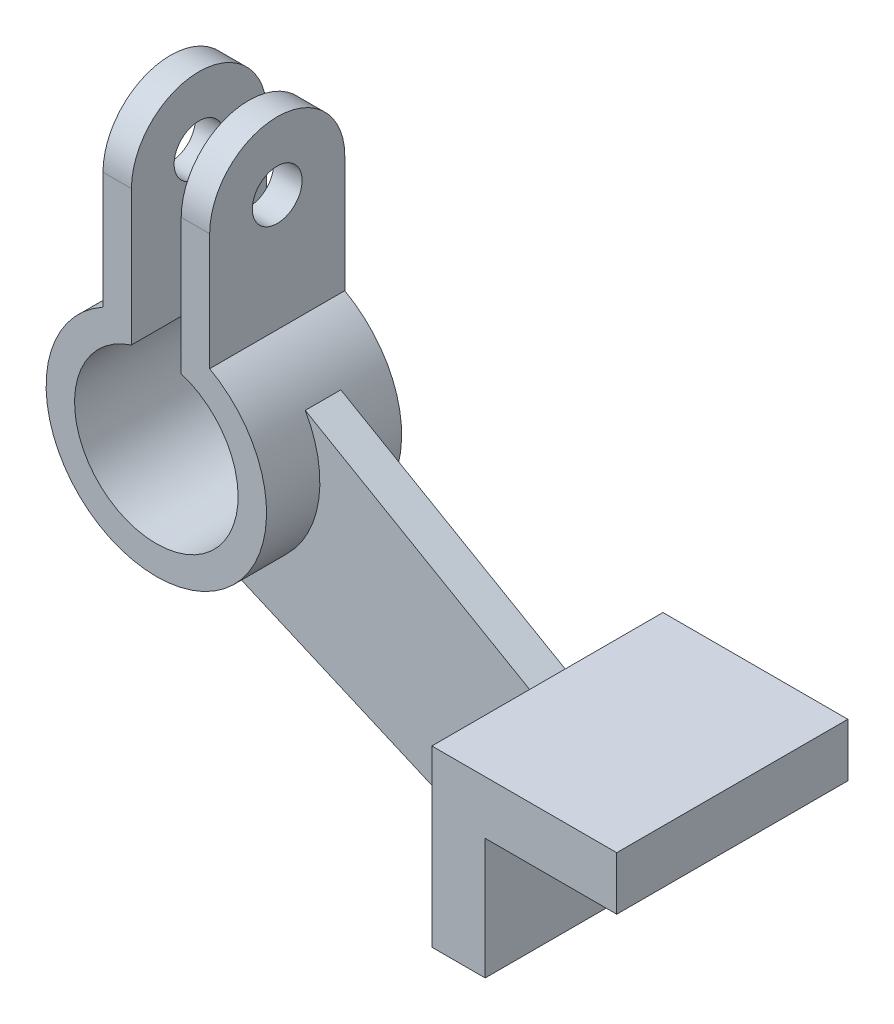
ISO-10303-21;
HEADER;
FILE_DESCRIPTION(('STEP AP214'),'2;1');
FILE_NAME('part.step','',(''),(''),'','','');
FILE_SCHEMA(('AUTOMOTIVE_DESIGN { 1 0 10303 214 1 1 1 1 }'));
ENDSEC;
DATA;
#1=APPLICATION_CONTEXT('core data for automotive mechanical design processes');
#2=APPLICATION_PROTOCOL_DEFINITION('international standard','automotive_design',2000,#1);
#3=PRODUCT_CONTEXT('',#1,'mechanical');
#4=PRODUCT('Part','Part','',(#3));
#5=PRODUCT_RELATED_PRODUCT_CATEGORY('part','',(#4));
#6=PRODUCT_DEFINITION_FORMATION('','',#4);
#7=PRODUCT_DEFINITION_CONTEXT('part definition',#1,'design');
#8=PRODUCT_DEFINITION('design','',#6,#7);
#9=PRODUCT_DEFINITION_SHAPE('','',#8);
#10=(LENGTH_UNIT() NAMED_UNIT(*) SI_UNIT(.MILLI.,.METRE.));
#11=(NAMED_UNIT(*) PLANE_ANGLE_UNIT() SI_UNIT($,.RADIAN.));
#12=(NAMED_UNIT(*) SI_UNIT($,.STERADIAN.) SOLID_ANGLE_UNIT());
#13=UNCERTAINTY_MEASURE_WITH_UNIT(LENGTH_MEASURE(1.E-05),#10,'distance_accuracy_value','');
#14=(GEOMETRIC_REPRESENTATION_CONTEXT(3) GLOBAL_UNCERTAINTY_ASSIGNED_CONTEXT((#13)) GLOBAL_UNIT_ASSIGNED_CONTEXT((#10,
#11,#12)) REPRESENTATION_CONTEXT('',''));
#15=CARTESIAN_POINT('',(0.,0.,0.));
#16=DIRECTION('',(0.,0.,1.));
#17=DIRECTION('',(1.,0.,0.));
#18=AXIS2_PLACEMENT_3D('',#15,#16,#17);
#19=CARTESIAN_POINT('',(-2.61943244872498E-13,1.4658413372004E-13,23.));
#20=DIRECTION('',(0.,0.,-1.));
#21=DIRECTION('',(-1.,0.,0.));
#22=AXIS2_PLACEMENT_3D('',#19,#20,#21);
#23=PLANE('',#22);
#24=DIRECTION('',(0.,-1.,0.));
#25=VECTOR('',#24,1.);
#26=CARTESIAN_POINT('',(90.,1.4658413372004E-13,23.));
#27=LINE('',#26,#25);
#28=CARTESIAN_POINT('',(90.,-21.0099338120634,23.));
#29=VERTEX_POINT('',#28);
#30=CARTESIAN_POINT('',(90.,-70.0360003093009,23.));
#31=VERTEX_POINT('',#30);
#32=EDGE_CURVE('E192',#29,#31,#27,.T.);
#33=ORIENTED_EDGE('',*,*,#32,.F.);
#34=DIRECTION('',(-0.86602540378444,0.499999999999998,0.));
#35=VECTOR('',#34,1.);
#36=CARTESIAN_POINT('',(90.,-21.0099338120634,23.));
#37=LINE('',#36,#35);
#38=CARTESIAN_POINT('',(26.888515956955,15.4274984891452,23.));
#39=VERTEX_POINT('',#38);
#40=EDGE_CURVE('E201',#29,#39,#37,.T.);
#41=ORIENTED_EDGE('',*,*,#40,.T.);
#42=CARTESIAN_POINT('',(-2.61943244872498E-13,1.4658413372004E-13,23.));
#43=DIRECTION('',(0.,0.,-1.));
#44=DIRECTION('',(-1.,0.,0.));
#45=AXIS2_PLACEMENT_3D('',#42,#43,#44);
#46=CIRCLE('',#45,31.0000000000002);
#47=CARTESIAN_POINT('',(0.,-31.,23.));
#48=VERTEX_POINT('',#47);
#49=EDGE_CURVE('E202',#39,#48,#46,.T.);
#50=ORIENTED_EDGE('',*,*,#49,.T.);
#51=DIRECTION('',(0.917421692084343,-0.397916371732931,0.));
#52=VECTOR('',#51,1.);
#53=CARTESIAN_POINT('',(90.,-70.0360003093009,23.));
#54=LINE('',#53,#52);
#55=EDGE_CURVE('E210',#48,#31,#54,.T.);
#56=ORIENTED_EDGE('',*,*,#55,.T.);
#57=EDGE_LOOP('',(#33,#41,#50,#56));
#58=FACE_BOUND('',#57,.T.);
#59=ADVANCED_FACE('F41',(#58),#23,.F.);
#60=CARTESIAN_POINT('',(-2.61943244872498E-13,1.4658413372004E-13,13.));
#61=DIRECTION('',(0.,0.,-1.));
#62=DIRECTION('',(-1.,0.,0.));
#63=AXIS2_PLACEMENT_3D('',#60,#61,#62);
#64=PLANE('',#63);
#65=DIRECTION('',(-0.86602540378444,0.499999999999998,0.));
#66=VECTOR('',#65,1.);
#67=CARTESIAN_POINT('',(90.,-21.0099338120634,13.));
#68=LINE('',#67,#66);
#69=CARTESIAN_POINT('',(90.,-21.0099338120634,13.));
#70=VERTEX_POINT('',#69);
#71=CARTESIAN_POINT('',(26.888515956955,15.4274984891452,13.));
#72=VERTEX_POINT('',#71);
#73=EDGE_CURVE('E197',#70,#72,#68,.T.);
#74=ORIENTED_EDGE('',*,*,#73,.F.);
#75=DIRECTION('',(0.,-1.,0.));
#76=VECTOR('',#75,1.);
#77=CARTESIAN_POINT('',(90.,1.4658413372004E-13,13.));
#78=LINE('',#77,#76);
#79=CARTESIAN_POINT('',(90.,-70.0360003093009,13.));
#80=VERTEX_POINT('',#79);
#81=EDGE_CURVE('E11',#70,#80,#78,.T.);
#82=ORIENTED_EDGE('',*,*,#81,.T.);
#83=DIRECTION('',(0.917421692084343,-0.397916371732931,0.));
#84=VECTOR('',#83,1.);
#85=CARTESIAN_POINT('',(90.,-70.0360003093009,13.));
#86=LINE('',#85,#84);
#87=CARTESIAN_POINT('',(0.,-31.,13.));
#88=VERTEX_POINT('',#87);
#89=EDGE_CURVE('E54',#88,#80,#86,.T.);
#90=ORIENTED_EDGE('',*,*,#89,.F.);
#91=CARTESIAN_POINT('',(-2.61943244872498E-13,1.4658413372004E-13,13.));
#92=DIRECTION('',(0.,0.,-1.));
#93=DIRECTION('',(-1.,0.,0.));
#94=AXIS2_PLACEMENT_3D('',#91,#92,#93);
#95=CIRCLE('',#94,31.0000000000002);
#96=EDGE_CURVE('E211',#72,#88,#95,.T.);
#97=ORIENTED_EDGE('',*,*,#96,.F.);
#98=EDGE_LOOP('',(#74,#82,#90,#97));
#99=FACE_BOUND('',#98,.T.);
#100=ADVANCED_FACE('F352',(#99),#64,.T.);
#101=CARTESIAN_POINT('',(0.,0.,38.));
#102=DIRECTION('',(0.,0.,-1.));
#103=DIRECTION('',(-1.,0.,0.));
#104=AXIS2_PLACEMENT_3D('',#101,#102,#103);
#105=CYLINDRICAL_SURFACE('',#104,31.);
#106=CARTESIAN_POINT('',(0.,0.,38.));
#107=DIRECTION('',(0.,0.,1.));
#108=DIRECTION('',(1.,0.,0.));
#109=AXIS2_PLACEMENT_3D('',#106,#107,#108);
#110=CIRCLE('',#109,31.);
#111=CARTESIAN_POINT('',(-15.,27.1293199325011,38.));
#112=VERTEX_POINT('',#111);
#113=CARTESIAN_POINT('',(15.,27.1293199325011,38.));
#114=VERTEX_POINT('',#113);
#115=EDGE_CURVE('E65',#112,#114,#110,.T.);
#116=ORIENTED_EDGE('',*,*,#115,.F.);
#117=DIRECTION('',(0.,0.,-1.));
#118=VECTOR('',#117,1.);
#119=CARTESIAN_POINT('',(-15.,27.1293199325011,38.));
#120=LINE('',#119,#118);
#121=CARTESIAN_POINT('',(-15.,27.1293199325011,0.));
#122=VERTEX_POINT('',#121);
#123=EDGE_CURVE('E47',#112,#122,#120,.T.);
#124=ORIENTED_EDGE('',*,*,#123,.T.);
#125=CARTESIAN_POINT('',(0.,0.,0.));
#126=DIRECTION('',(0.,0.,1.));
#127=DIRECTION('',(1.,0.,0.));
#128=AXIS2_PLACEMENT_3D('',#125,#126,#127);
#129=CIRCLE('',#128,31.);
#130=CARTESIAN_POINT('',(15.,27.1293199325011,0.));
#131=VERTEX_POINT('',#130);
#132=EDGE_CURVE('E289',#122,#131,#129,.T.);
#133=ORIENTED_EDGE('',*,*,#132,.T.);
#134=DIRECTION('',(0.,0.,-1.));
#135=VECTOR('',#134,1.);
#136=CARTESIAN_POINT('',(15.,27.1293199325011,38.));
#137=LINE('',#136,#135);
#138=EDGE_CURVE('E296',#131,#114,#137,.F.);
#139=ORIENTED_EDGE('',*,*,#138,.T.);
#140=EDGE_LOOP('',(#116,#124,#133,#139));
#141=FACE_BOUND('',#140,.T.);
#142=ORIENTED_EDGE('',*,*,#49,.F.);
#143=DIRECTION('',(0.,0.,-1.));
#144=VECTOR('',#143,1.);
#145=CARTESIAN_POINT('',(26.888515956955,15.4274984891452,23.));
#146=LINE('',#145,#144);
#147=EDGE_CURVE('E217',#39,#72,#146,.T.);
#148=ORIENTED_EDGE('',*,*,#147,.T.);
#149=ORIENTED_EDGE('',*,*,#96,.T.);
#150=DIRECTION('',(0.,0.,-1.));
#151=VECTOR('',#150,1.);
#152=CARTESIAN_POINT('',(0.,-31.,23.));
#153=LINE('',#152,#151);
#154=EDGE_CURVE('E216',#48,#88,#153,.T.);
#155=ORIENTED_EDGE('',*,*,#154,.F.);
#156=EDGE_LOOP('',(#142,#148,#149,#155));
#157=FACE_BOUND('',#156,.T.);
#158=ADVANCED_FACE('F43',(#141,#157),#105,.T.);
#159=CARTESIAN_POINT('',(0.,0.,38.));
#160=DIRECTION('',(0.,0.,1.));
#161=DIRECTION('',(1.,0.,0.));
#162=AXIS2_PLACEMENT_3D('',#159,#160,#161);
#163=PLANE('',#162);
#164=CARTESIAN_POINT('',(0.,0.,38.));
#165=DIRECTION('',(0.,0.,1.));
#166=DIRECTION('',(1.,0.,0.));
#167=AXIS2_PLACEMENT_3D('',#164,#165,#166);
#168=CIRCLE('',#167,23.);
#169=CARTESIAN_POINT('',(-7.,21.9089023002066,38.));
#170=VERTEX_POINT('',#169);
#171=CARTESIAN_POINT('',(7.,21.9089023002066,38.));
#172=VERTEX_POINT('',#171);
#173=EDGE_CURVE('E290',#170,#172,#168,.T.);
#174=ORIENTED_EDGE('',*,*,#173,.F.);
#175=DIRECTION('',(0.,-1.,0.));
#176=VECTOR('',#175,1.);
#177=CARTESIAN_POINT('',(-7.,0.,38.));
#178=LINE('',#177,#176);
#179=CARTESIAN_POINT('',(-7.,60.,38.));
#180=VERTEX_POINT('',#179);
#181=EDGE_CURVE('E282',#180,#170,#178,.T.);
#182=ORIENTED_EDGE('',*,*,#181,.F.);
#183=DIRECTION('',(1.,0.,0.));
#184=VECTOR('',#183,1.);
#185=CARTESIAN_POINT('',(-15.,60.,38.));
#186=LINE('',#185,#184);
#187=CARTESIAN_POINT('',(-15.,60.,38.));
#188=VERTEX_POINT('',#187);
#189=EDGE_CURVE('E248',#188,#180,#186,.T.);
#190=ORIENTED_EDGE('',*,*,#189,.F.);
#191=DIRECTION('',(0.,-1.,0.));
#192=VECTOR('',#191,1.);
#193=CARTESIAN_POINT('',(-15.,60.,38.));
#194=LINE('',#193,#192);
#195=EDGE_CURVE('E245',#188,#112,#194,.T.);
#196=ORIENTED_EDGE('',*,*,#195,.T.);
#197=ORIENTED_EDGE('',*,*,#115,.T.);
#198=DIRECTION('',(0.,-1.,0.));
#199=VECTOR('',#198,1.);
#200=CARTESIAN_POINT('',(15.,60.,38.));
#201=LINE('',#200,#199);
#202=CARTESIAN_POINT('',(15.,60.,38.));
#203=VERTEX_POINT('',#202);
#204=EDGE_CURVE('E262',#203,#114,#201,.T.);
#205=ORIENTED_EDGE('',*,*,#204,.F.);
#206=DIRECTION('',(-1.,0.,0.));
#207=VECTOR('',#206,1.);
#208=CARTESIAN_POINT('',(15.,60.,38.));
#209=LINE('',#208,#207);
#210=CARTESIAN_POINT('',(7.,60.,38.));
#211=VERTEX_POINT('',#210);
#212=EDGE_CURVE('E273',#203,#211,#209,.T.);
#213=ORIENTED_EDGE('',*,*,#212,.T.);
#214=DIRECTION('',(0.,1.,0.));
#215=VECTOR('',#214,1.);
#216=CARTESIAN_POINT('',(7.,0.,38.));
#217=LINE('',#216,#215);
#218=EDGE_CURVE('E280',#172,#211,#217,.T.);
#219=ORIENTED_EDGE('',*,*,#218,.F.);
#220=EDGE_LOOP('',(#174,#182,#190,#196,#197,#205,#213,#219));
#221=FACE_BOUND('',#220,.T.);
#222=ADVANCED_FACE('F328',(#221),#163,.T.);
#223=CARTESIAN_POINT('',(0.,0.,0.));
#224=DIRECTION('',(0.,0.,1.));
#225=DIRECTION('',(1.,0.,0.));
#226=AXIS2_PLACEMENT_3D('',#223,#224,#225);
#227=PLANE('',#226);
#228=DIRECTION('',(0.,-1.,0.));
#229=VECTOR('',#228,1.);
#230=CARTESIAN_POINT('',(-7.,0.,0.));
#231=LINE('',#230,#229);
#232=CARTESIAN_POINT('',(-7.,60.,0.));
#233=VERTEX_POINT('',#232);
#234=CARTESIAN_POINT('',(-7.,21.9089023002066,0.));
#235=VERTEX_POINT('',#234);
#236=EDGE_CURVE('E278',#233,#235,#231,.T.);
#237=ORIENTED_EDGE('',*,*,#236,.T.);
#238=CARTESIAN_POINT('',(0.,0.,0.));
#239=DIRECTION('',(0.,0.,1.));
#240=DIRECTION('',(1.,0.,0.));
#241=AXIS2_PLACEMENT_3D('',#238,#239,#240);
#242=CIRCLE('',#241,23.);
#243=CARTESIAN_POINT('',(7.,21.9089023002066,0.));
#244=VERTEX_POINT('',#243);
#245=EDGE_CURVE('E281',#235,#244,#242,.T.);
#246=ORIENTED_EDGE('',*,*,#245,.T.);
#247=DIRECTION('',(0.,1.,0.));
#248=VECTOR('',#247,1.);
#249=CARTESIAN_POINT('',(7.,0.,0.));
#250=LINE('',#249,#248);
#251=CARTESIAN_POINT('',(7.,60.,0.));
#252=VERTEX_POINT('',#251);
#253=EDGE_CURVE('E279',#244,#252,#250,.T.);
#254=ORIENTED_EDGE('',*,*,#253,.T.);
#255=DIRECTION('',(-1.,0.,0.));
#256=VECTOR('',#255,1.);
#257=CARTESIAN_POINT('',(15.,60.,0.));
#258=LINE('',#257,#256);
#259=CARTESIAN_POINT('',(15.,60.,0.));
#260=VERTEX_POINT('',#259);
#261=EDGE_CURVE('E267',#260,#252,#258,.T.);
#262=ORIENTED_EDGE('',*,*,#261,.F.);
#263=DIRECTION('',(0.,1.,0.));
#264=VECTOR('',#263,1.);
#265=CARTESIAN_POINT('',(15.,21.9089023002066,0.));
#266=LINE('',#265,#264);
#267=EDGE_CURVE('E270',#131,#260,#266,.T.);
#268=ORIENTED_EDGE('',*,*,#267,.F.);
#269=ORIENTED_EDGE('',*,*,#132,.F.);
#270=DIRECTION('',(0.,1.,0.));
#271=VECTOR('',#270,1.);
#272=CARTESIAN_POINT('',(-15.,21.9089023002066,0.));
#273=LINE('',#272,#271);
#274=CARTESIAN_POINT('',(-15.,60.,0.));
#275=VERTEX_POINT('',#274);
#276=EDGE_CURVE('E242',#122,#275,#273,.T.);
#277=ORIENTED_EDGE('',*,*,#276,.T.);
#278=DIRECTION('',(1.,0.,0.));
#279=VECTOR('',#278,1.);
#280=CARTESIAN_POINT('',(-15.,60.,0.));
#281=LINE('',#280,#279);
#282=EDGE_CURVE('E253',#275,#233,#281,.T.);
#283=ORIENTED_EDGE('',*,*,#282,.T.);
#284=EDGE_LOOP('',(#237,#246,#254,#262,#268,#269,#277,#283));
#285=FACE_BOUND('',#284,.T.);
#286=ADVANCED_FACE('F306',(#285),#227,.F.);
#287=CARTESIAN_POINT('',(0.,0.,38.));
#288=DIRECTION('',(0.,0.,-1.));
#289=DIRECTION('',(-1.,0.,0.));
#290=AXIS2_PLACEMENT_3D('',#287,#288,#289);
#291=CYLINDRICAL_SURFACE('',#290,23.);
#292=DIRECTION('',(0.,0.,-1.));
#293=VECTOR('',#292,1.);
#294=CARTESIAN_POINT('',(-7.,21.9089023002066,38.));
#295=LINE('',#294,#293);
#296=EDGE_CURVE('E299',#170,#235,#295,.T.);
#297=ORIENTED_EDGE('',*,*,#296,.F.);
#298=ORIENTED_EDGE('',*,*,#173,.T.);
#299=DIRECTION('',(0.,0.,-1.));
#300=VECTOR('',#299,1.);
#301=CARTESIAN_POINT('',(7.,21.9089023002066,38.));
#302=LINE('',#301,#300);
#303=EDGE_CURVE('E294',#244,#172,#302,.F.);
#304=ORIENTED_EDGE('',*,*,#303,.F.);
#305=ORIENTED_EDGE('',*,*,#245,.F.);
#306=EDGE_LOOP('',(#297,#298,#304,#305));
#307=FACE_BOUND('',#306,.T.);
#308=ADVANCED_FACE('F321',(#307),#291,.F.);
#309=CARTESIAN_POINT('',(7.,0.,0.));
#310=DIRECTION('',(1.,0.,0.));
#311=DIRECTION('',(0.,0.,-1.));
#312=AXIS2_PLACEMENT_3D('',#309,#310,#311);
#313=PLANE('',#312);
#314=ORIENTED_EDGE('',*,*,#253,.F.);
#315=ORIENTED_EDGE('',*,*,#303,.T.);
#316=ORIENTED_EDGE('',*,*,#218,.T.);
#317=CARTESIAN_POINT('',(7.,60.,19.));
#318=DIRECTION('',(1.,0.,0.));
#319=DIRECTION('',(0.,0.,-1.));
#320=AXIS2_PLACEMENT_3D('',#317,#318,#319);
#321=CIRCLE('',#320,19.);
#322=EDGE_CURVE('E256',#252,#211,#321,.T.);
#323=ORIENTED_EDGE('',*,*,#322,.F.);
#324=EDGE_LOOP('',(#314,#315,#316,#323));
#325=FACE_BOUND('',#324,.T.);
#326=CARTESIAN_POINT('',(7.,60.,19.));
#327=DIRECTION('',(1.,0.,0.));
#328=DIRECTION('',(0.,0.,-1.));
#329=AXIS2_PLACEMENT_3D('',#326,#327,#328);
#330=CIRCLE('',#329,7.);
#331=CARTESIAN_POINT('',(7.,60.,12.));
#332=VERTEX_POINT('',#331);
#333=EDGE_CURVE('E255',#332,#332,#330,.T.);
#334=ORIENTED_EDGE('',*,*,#333,.T.);
#335=EDGE_LOOP('',(#334));
#336=FACE_BOUND('',#335,.T.);
#337=ADVANCED_FACE('F324',(#325,#336),#313,.F.);
#338=CARTESIAN_POINT('',(-7.,0.,0.));
#339=DIRECTION('',(-1.,0.,0.));
#340=DIRECTION('',(0.,0.,1.));
#341=AXIS2_PLACEMENT_3D('',#338,#339,#340);
#342=PLANE('',#341);
#343=ORIENTED_EDGE('',*,*,#181,.T.);
#344=ORIENTED_EDGE('',*,*,#296,.T.);
#345=ORIENTED_EDGE('',*,*,#236,.F.);
#346=CARTESIAN_POINT('',(-7.,60.,19.));
#347=DIRECTION('',(1.,0.,0.));
#348=DIRECTION('',(0.,0.,-1.));
#349=AXIS2_PLACEMENT_3D('',#346,#347,#348);
#350=CIRCLE('',#349,19.);
#351=EDGE_CURVE('E234',#233,#180,#350,.T.);
#352=ORIENTED_EDGE('',*,*,#351,.T.);
#353=EDGE_LOOP('',(#343,#344,#345,#352));
#354=FACE_BOUND('',#353,.T.);
#355=CARTESIAN_POINT('',(-7.,60.,19.));
#356=DIRECTION('',(1.,0.,0.));
#357=DIRECTION('',(0.,0.,-1.));
#358=AXIS2_PLACEMENT_3D('',#355,#356,#357);
#359=CIRCLE('',#358,7.);
#360=CARTESIAN_POINT('',(-7.,60.,12.));
#361=VERTEX_POINT('',#360);
#362=EDGE_CURVE('E233',#361,#361,#359,.T.);
#363=ORIENTED_EDGE('',*,*,#362,.F.);
#364=EDGE_LOOP('',(#363));
#365=FACE_BOUND('',#364,.T.);
#366=ADVANCED_FACE('F339',(#354,#365),#342,.F.);
#367=CARTESIAN_POINT('',(15.,60.,19.));
#368=DIRECTION('',(1.,0.,0.));
#369=DIRECTION('',(0.,0.,-1.));
#370=AXIS2_PLACEMENT_3D('',#367,#368,#369);
#371=PLANE('',#370);
#372=CARTESIAN_POINT('',(15.,60.,19.));
#373=DIRECTION('',(1.,0.,0.));
#374=DIRECTION('',(0.,0.,-1.));
#375=AXIS2_PLACEMENT_3D('',#372,#373,#374);
#376=CIRCLE('',#375,7.);
#377=CARTESIAN_POINT('',(15.,60.,12.));
#378=VERTEX_POINT('',#377);
#379=EDGE_CURVE('E254',#378,#378,#376,.T.);
#380=ORIENTED_EDGE('',*,*,#379,.F.);
#381=EDGE_LOOP('',(#380));
#382=FACE_BOUND('',#381,.T.);
#383=ORIENTED_EDGE('',*,*,#138,.F.);
#384=ORIENTED_EDGE('',*,*,#267,.T.);
#385=CARTESIAN_POINT('',(15.,60.,19.));
#386=DIRECTION('',(1.,0.,0.));
#387=DIRECTION('',(0.,0.,-1.));
#388=AXIS2_PLACEMENT_3D('',#385,#386,#387);
#389=CIRCLE('',#388,19.);
#390=EDGE_CURVE('E261',#260,#203,#389,.T.);
#391=ORIENTED_EDGE('',*,*,#390,.T.);
#392=ORIENTED_EDGE('',*,*,#204,.T.);
#393=EDGE_LOOP('',(#383,#384,#391,#392));
#394=FACE_BOUND('',#393,.T.);
#395=ADVANCED_FACE('F333',(#382,#394),#371,.T.);
#396=CARTESIAN_POINT('',(15.,60.,19.));
#397=DIRECTION('',(-1.,0.,0.));
#398=DIRECTION('',(0.,0.,1.));
#399=AXIS2_PLACEMENT_3D('',#396,#397,#398);
#400=CYLINDRICAL_SURFACE('',#399,19.);
#401=ORIENTED_EDGE('',*,*,#322,.T.);
#402=ORIENTED_EDGE('',*,*,#212,.F.);
#403=ORIENTED_EDGE('',*,*,#390,.F.);
#404=ORIENTED_EDGE('',*,*,#261,.T.);
#405=EDGE_LOOP('',(#401,#402,#403,#404));
#406=FACE_BOUND('',#405,.T.);
#407=ADVANCED_FACE('F334',(#406),#400,.T.);
#408=CARTESIAN_POINT('',(15.,60.,19.));
#409=DIRECTION('',(-1.,0.,0.));
#410=DIRECTION('',(0.,0.,1.));
#411=AXIS2_PLACEMENT_3D('',#408,#409,#410);
#412=CYLINDRICAL_SURFACE('',#411,7.);
#413=ORIENTED_EDGE('',*,*,#379,.T.);
#414=EDGE_LOOP('',(#413));
#415=FACE_BOUND('',#414,.T.);
#416=ORIENTED_EDGE('',*,*,#333,.F.);
#417=EDGE_LOOP('',(#416));
#418=FACE_BOUND('',#417,.T.);
#419=ADVANCED_FACE('F342',(#415,#418),#412,.F.);
#420=CARTESIAN_POINT('',(-15.,60.,19.));
#421=DIRECTION('',(-1.,0.,0.));
#422=DIRECTION('',(0.,0.,-1.));
#423=AXIS2_PLACEMENT_3D('',#420,#421,#422);
#424=PLANE('',#423);
#425=CARTESIAN_POINT('',(-15.,60.,19.));
#426=DIRECTION('',(1.,0.,0.));
#427=DIRECTION('',(0.,0.,-1.));
#428=AXIS2_PLACEMENT_3D('',#425,#426,#427);
#429=CIRCLE('',#428,7.);
#430=CARTESIAN_POINT('',(-15.,60.,12.));
#431=VERTEX_POINT('',#430);
#432=EDGE_CURVE('E235',#431,#431,#429,.T.);
#433=ORIENTED_EDGE('',*,*,#432,.T.);
#434=EDGE_LOOP('',(#433));
#435=FACE_BOUND('',#434,.T.);
#436=ORIENTED_EDGE('',*,*,#123,.F.);
#437=ORIENTED_EDGE('',*,*,#195,.F.);
#438=CARTESIAN_POINT('',(-15.,60.,19.));
#439=DIRECTION('',(1.,0.,0.));
#440=DIRECTION('',(0.,0.,-1.));
#441=AXIS2_PLACEMENT_3D('',#438,#439,#440);
#442=CIRCLE('',#441,19.);
#443=EDGE_CURVE('E236',#275,#188,#442,.T.);
#444=ORIENTED_EDGE('',*,*,#443,.F.);
#445=ORIENTED_EDGE('',*,*,#276,.F.);
#446=EDGE_LOOP('',(#436,#437,#444,#445));
#447=FACE_BOUND('',#446,.T.);
#448=ADVANCED_FACE('F315',(#435,#447),#424,.T.);
#449=CARTESIAN_POINT('',(-15.,60.,19.));
#450=DIRECTION('',(1.,0.,0.));
#451=DIRECTION('',(0.,0.,-1.));
#452=AXIS2_PLACEMENT_3D('',#449,#450,#451);
#453=CYLINDRICAL_SURFACE('',#452,19.);
#454=ORIENTED_EDGE('',*,*,#351,.F.);
#455=ORIENTED_EDGE('',*,*,#282,.F.);
#456=ORIENTED_EDGE('',*,*,#443,.T.);
#457=ORIENTED_EDGE('',*,*,#189,.T.);
#458=EDGE_LOOP('',(#454,#455,#456,#457));
#459=FACE_BOUND('',#458,.T.);
#460=ADVANCED_FACE('F312',(#459),#453,.T.);
#461=CARTESIAN_POINT('',(-15.,60.,19.));
#462=DIRECTION('',(1.,0.,0.));
#463=DIRECTION('',(0.,0.,-1.));
#464=AXIS2_PLACEMENT_3D('',#461,#462,#463);
#465=CYLINDRICAL_SURFACE('',#464,7.);
#466=ORIENTED_EDGE('',*,*,#432,.F.);
#467=EDGE_LOOP('',(#466));
#468=FACE_BOUND('',#467,.T.);
#469=ORIENTED_EDGE('',*,*,#362,.T.);
#470=EDGE_LOOP('',(#469));
#471=FACE_BOUND('',#470,.T.);
#472=ADVANCED_FACE('F388',(#468,#471),#465,.F.);
#473=CARTESIAN_POINT('',(90.,-70.0360003093009,23.));
#474=DIRECTION('',(0.,1.,0.));
#475=DIRECTION('',(0.,0.,1.));
#476=AXIS2_PLACEMENT_3D('',#473,#474,#475);
#477=PLANE('',#476);
#478=DIRECTION('',(0.,0.,-1.));
#479=VECTOR('',#478,1.);
#480=CARTESIAN_POINT('',(90.,-70.0360003093009,23.));
#481=LINE('',#480,#479);
#482=EDGE_CURVE('E207',#31,#80,#481,.T.);
#483=ORIENTED_EDGE('',*,*,#482,.T.);
#484=DIRECTION('',(0.,0.,-1.));
#485=VECTOR('',#484,1.);
#486=CARTESIAN_POINT('',(90.,-70.0360003093009,50.5));
#487=LINE('',#486,#485);
#488=CARTESIAN_POINT('',(90.,-70.0360003093009,-14.5));
#489=VERTEX_POINT('',#488);
#490=EDGE_CURVE('E194',#80,#489,#487,.T.);
#491=ORIENTED_EDGE('',*,*,#490,.T.);
#492=DIRECTION('',(1.,0.,0.));
#493=VECTOR('',#492,1.);
#494=CARTESIAN_POINT('',(90.,-70.0360003093009,-14.5));
#495=LINE('',#494,#493);
#496=CARTESIAN_POINT('',(105.,-70.0360003093009,-14.5));
#497=VERTEX_POINT('',#496);
#498=EDGE_CURVE('E555',#489,#497,#495,.T.);
#499=ORIENTED_EDGE('',*,*,#498,.T.);
#500=DIRECTION('',(0.,0.,-1.));
#501=VECTOR('',#500,1.);
#502=CARTESIAN_POINT('',(105.,-70.0360003093009,23.));
#503=LINE('',#502,#501);
#504=CARTESIAN_POINT('',(105.,-70.0360003093009,50.5));
#505=VERTEX_POINT('',#504);
#506=EDGE_CURVE('E171',#505,#497,#503,.T.);
#507=ORIENTED_EDGE('',*,*,#506,.F.);
#508=DIRECTION('',(1.,0.,0.));
#509=VECTOR('',#508,1.);
#510=CARTESIAN_POINT('',(90.,-70.0360003093009,50.5));
#511=LINE('',#510,#509);
#512=CARTESIAN_POINT('',(90.,-70.0360003093009,50.5));
#513=VERTEX_POINT('',#512);
#514=EDGE_CURVE('E170',#513,#505,#511,.T.);
#515=ORIENTED_EDGE('',*,*,#514,.F.);
#516=EDGE_CURVE('E174',#513,#31,#487,.T.);
#517=ORIENTED_EDGE('',*,*,#516,.T.);
#518=EDGE_LOOP('',(#483,#491,#499,#507,#515,#517));
#519=FACE_BOUND('',#518,.T.);
#520=ADVANCED_FACE('F168',(#519),#477,.F.);
#521=CARTESIAN_POINT('',(105.,-70.0360003093009,23.));
#522=DIRECTION('',(-1.,0.,0.));
#523=DIRECTION('',(0.,-1.,0.));
#524=AXIS2_PLACEMENT_3D('',#521,#522,#523);
#525=PLANE('',#524);
#526=ORIENTED_EDGE('',*,*,#506,.T.);
#527=DIRECTION('',(0.,1.,0.));
#528=VECTOR('',#527,1.);
#529=CARTESIAN_POINT('',(105.,-36.0099338120634,-14.5));
#530=LINE('',#529,#528);
#531=CARTESIAN_POINT('',(105.,-36.0099338120634,-14.5));
#532=VERTEX_POINT('',#531);
#533=EDGE_CURVE('E551',#497,#532,#530,.T.);
#534=ORIENTED_EDGE('',*,*,#533,.T.);
#535=DIRECTION('',(0.,0.,-1.));
#536=VECTOR('',#535,1.);
#537=CARTESIAN_POINT('',(105.,-36.0099338120634,23.));
#538=LINE('',#537,#536);
#539=CARTESIAN_POINT('',(105.,-36.0099338120634,50.5));
#540=VERTEX_POINT('',#539);
#541=EDGE_CURVE('E230',#540,#532,#538,.T.);
#542=ORIENTED_EDGE('',*,*,#541,.F.);
#543=DIRECTION('',(0.,1.,0.));
#544=VECTOR('',#543,1.);
#545=CARTESIAN_POINT('',(105.,-36.0099338120634,50.5));
#546=LINE('',#545,#544);
#547=EDGE_CURVE('E176',#505,#540,#546,.T.);
#548=ORIENTED_EDGE('',*,*,#547,.F.);
#549=EDGE_LOOP('',(#526,#534,#542,#548));
#550=FACE_BOUND('',#549,.T.);
#551=ADVANCED_FACE('F382',(#550),#525,.F.);
#552=CARTESIAN_POINT('',(105.,-36.0099338120634,23.));
#553=DIRECTION('',(0.,1.,0.));
#554=DIRECTION('',(-1.,0.,0.));
#555=AXIS2_PLACEMENT_3D('',#552,#553,#554);
#556=PLANE('',#555);
#557=ORIENTED_EDGE('',*,*,#541,.T.);
#558=DIRECTION('',(1.,0.,0.));
#559=VECTOR('',#558,1.);
#560=CARTESIAN_POINT('',(142.,-36.0099338120634,-14.5));
#561=LINE('',#560,#559);
#562=CARTESIAN_POINT('',(142.,-36.0099338120634,-14.5));
#563=VERTEX_POINT('',#562);
#564=EDGE_CURVE('E563',#532,#563,#561,.T.);
#565=ORIENTED_EDGE('',*,*,#564,.T.);
#566=DIRECTION('',(0.,0.,-1.));
#567=VECTOR('',#566,1.);
#568=CARTESIAN_POINT('',(142.,-36.0099338120634,23.));
#569=LINE('',#568,#567);
#570=CARTESIAN_POINT('',(142.,-36.0099338120634,50.5));
#571=VERTEX_POINT('',#570);
#572=EDGE_CURVE('E227',#571,#563,#569,.T.);
#573=ORIENTED_EDGE('',*,*,#572,.F.);
#574=DIRECTION('',(1.,0.,0.));
#575=VECTOR('',#574,1.);
#576=CARTESIAN_POINT('',(142.,-36.0099338120634,50.5));
#577=LINE('',#576,#575);
#578=EDGE_CURVE('E575',#540,#571,#577,.T.);
#579=ORIENTED_EDGE('',*,*,#578,.F.);
#580=EDGE_LOOP('',(#557,#565,#573,#579));
#581=FACE_BOUND('',#580,.T.);
#582=ADVANCED_FACE('F377',(#581),#556,.F.);
#583=CARTESIAN_POINT('',(142.,-36.0099338120634,23.));
#584=DIRECTION('',(-1.,0.,0.));
#585=DIRECTION('',(0.,-1.,0.));
#586=AXIS2_PLACEMENT_3D('',#583,#584,#585);
#587=PLANE('',#586);
#588=ORIENTED_EDGE('',*,*,#572,.T.);
#589=DIRECTION('',(0.,1.,0.));
#590=VECTOR('',#589,1.);
#591=CARTESIAN_POINT('',(142.,-21.0099338120634,-14.5));
#592=LINE('',#591,#590);
#593=CARTESIAN_POINT('',(142.,-21.0099338120634,-14.5));
#594=VERTEX_POINT('',#593);
#595=EDGE_CURVE('E562',#563,#594,#592,.T.);
#596=ORIENTED_EDGE('',*,*,#595,.T.);
#597=DIRECTION('',(0.,0.,-1.));
#598=VECTOR('',#597,1.);
#599=CARTESIAN_POINT('',(142.,-21.0099338120634,23.));
#600=LINE('',#599,#598);
#601=CARTESIAN_POINT('',(142.,-21.0099338120634,50.5));
#602=VERTEX_POINT('',#601);
#603=EDGE_CURVE('E221',#602,#594,#600,.T.);
#604=ORIENTED_EDGE('',*,*,#603,.F.);
#605=DIRECTION('',(0.,1.,0.));
#606=VECTOR('',#605,1.);
#607=CARTESIAN_POINT('',(142.,-21.0099338120634,50.5));
#608=LINE('',#607,#606);
#609=EDGE_CURVE('E579',#571,#602,#608,.T.);
#610=ORIENTED_EDGE('',*,*,#609,.F.);
#611=EDGE_LOOP('',(#588,#596,#604,#610));
#612=FACE_BOUND('',#611,.T.);
#613=ADVANCED_FACE('F374',(#612),#587,.F.);
#614=CARTESIAN_POINT('',(142.,-21.0099338120634,23.));
#615=DIRECTION('',(0.,-1.,0.));
#616=DIRECTION('',(1.,0.,0.));
#617=AXIS2_PLACEMENT_3D('',#614,#615,#616);
#618=PLANE('',#617);
#619=ORIENTED_EDGE('',*,*,#603,.T.);
#620=DIRECTION('',(-1.,0.,0.));
#621=VECTOR('',#620,1.);
#622=CARTESIAN_POINT('',(90.,-21.0099338120634,-14.5));
#623=LINE('',#622,#621);
#624=CARTESIAN_POINT('',(90.,-21.0099338120634,-14.5));
#625=VERTEX_POINT('',#624);
#626=EDGE_CURVE('E186',#594,#625,#623,.T.);
#627=ORIENTED_EDGE('',*,*,#626,.T.);
#628=DIRECTION('',(0.,0.,-1.));
#629=VECTOR('',#628,1.);
#630=CARTESIAN_POINT('',(90.,-21.0099338120634,50.5));
#631=LINE('',#630,#629);
#632=EDGE_CURVE('E570',#70,#625,#631,.T.);
#633=ORIENTED_EDGE('',*,*,#632,.F.);
#634=DIRECTION('',(0.,0.,-1.));
#635=VECTOR('',#634,1.);
#636=CARTESIAN_POINT('',(90.,-21.0099338120634,23.));
#637=LINE('',#636,#635);
#638=EDGE_CURVE('E222',#29,#70,#637,.T.);
#639=ORIENTED_EDGE('',*,*,#638,.F.);
#640=CARTESIAN_POINT('',(90.,-21.0099338120634,50.5));
#641=VERTEX_POINT('',#640);
#642=EDGE_CURVE('E200',#641,#29,#631,.T.);
#643=ORIENTED_EDGE('',*,*,#642,.F.);
#644=DIRECTION('',(-1.,0.,0.));
#645=VECTOR('',#644,1.);
#646=CARTESIAN_POINT('',(90.,-21.0099338120634,50.5));
#647=LINE('',#646,#645);
#648=EDGE_CURVE('E183',#602,#641,#647,.T.);
#649=ORIENTED_EDGE('',*,*,#648,.F.);
#650=EDGE_LOOP('',(#619,#627,#633,#639,#643,#649));
#651=FACE_BOUND('',#650,.T.);
#652=ADVANCED_FACE('F371',(#651),#618,.F.);
#653=CARTESIAN_POINT('',(90.,-21.0099338120634,23.));
#654=DIRECTION('',(-0.499999999999998,-0.86602540378444,0.));
#655=DIRECTION('',(0.86602540378444,-0.499999999999998,0.));
#656=AXIS2_PLACEMENT_3D('',#653,#654,#655);
#657=PLANE('',#656);
#658=ORIENTED_EDGE('',*,*,#73,.T.);
#659=ORIENTED_EDGE('',*,*,#147,.F.);
#660=ORIENTED_EDGE('',*,*,#40,.F.);
#661=ORIENTED_EDGE('',*,*,#638,.T.);
#662=EDGE_LOOP('',(#658,#659,#660,#661));
#663=FACE_BOUND('',#662,.T.);
#664=ADVANCED_FACE('F370',(#663),#657,.F.);
#665=CARTESIAN_POINT('',(90.,-70.0360003093009,23.));
#666=DIRECTION('',(0.397916371732931,0.917421692084343,0.));
#667=DIRECTION('',(-0.917421692084343,0.397916371732931,0.));
#668=AXIS2_PLACEMENT_3D('',#665,#666,#667);
#669=PLANE('',#668);
#670=ORIENTED_EDGE('',*,*,#89,.T.);
#671=ORIENTED_EDGE('',*,*,#482,.F.);
#672=ORIENTED_EDGE('',*,*,#55,.F.);
#673=ORIENTED_EDGE('',*,*,#154,.T.);
#674=EDGE_LOOP('',(#670,#671,#672,#673));
#675=FACE_BOUND('',#674,.T.);
#676=ADVANCED_FACE('F361',(#675),#669,.F.);
#677=CARTESIAN_POINT('',(0.,0.,-14.5));
#678=DIRECTION('',(0.,0.,-1.));
#679=DIRECTION('',(-1.,0.,0.));
#680=AXIS2_PLACEMENT_3D('',#677,#678,#679);
#681=PLANE('',#680);
#682=DIRECTION('',(0.,-1.,0.));
#683=VECTOR('',#682,1.);
#684=CARTESIAN_POINT('',(90.,-70.0360003093009,-14.5));
#685=LINE('',#684,#683);
#686=EDGE_CURVE('E547',#625,#489,#685,.T.);
#687=ORIENTED_EDGE('',*,*,#686,.F.);
#688=ORIENTED_EDGE('',*,*,#626,.F.);
#689=ORIENTED_EDGE('',*,*,#595,.F.);
#690=ORIENTED_EDGE('',*,*,#564,.F.);
#691=ORIENTED_EDGE('',*,*,#533,.F.);
#692=ORIENTED_EDGE('',*,*,#498,.F.);
#693=EDGE_LOOP('',(#687,#688,#689,#690,#691,#692));
#694=FACE_BOUND('',#693,.T.);
#695=ADVANCED_FACE('F368',(#694),#681,.T.);
#696=CARTESIAN_POINT('',(90.,-70.0360003093009,50.5));
#697=DIRECTION('',(1.,0.,0.));
#698=DIRECTION('',(0.,0.,-1.));
#699=AXIS2_PLACEMENT_3D('',#696,#697,#698);
#700=PLANE('',#699);
#701=ORIENTED_EDGE('',*,*,#81,.F.);
#702=ORIENTED_EDGE('',*,*,#632,.T.);
#703=ORIENTED_EDGE('',*,*,#686,.T.);
#704=ORIENTED_EDGE('',*,*,#490,.F.);
#705=EDGE_LOOP('',(#701,#702,#703,#704));
#706=FACE_BOUND('',#705,.T.);
#707=ADVANCED_FACE('F359',(#706),#700,.F.);
#708=ORIENTED_EDGE('',*,*,#642,.T.);
#709=ORIENTED_EDGE('',*,*,#32,.T.);
#710=ORIENTED_EDGE('',*,*,#516,.F.);
#711=DIRECTION('',(0.,-1.,0.));
#712=VECTOR('',#711,1.);
#713=CARTESIAN_POINT('',(90.,-70.0360003093009,50.5));
#714=LINE('',#713,#712);
#715=EDGE_CURVE('E177',#641,#513,#714,.T.);
#716=ORIENTED_EDGE('',*,*,#715,.F.);
#717=EDGE_LOOP('',(#708,#709,#710,#716));
#718=FACE_BOUND('',#717,.T.);
#719=ADVANCED_FACE('F195',(#718),#700,.F.);
#720=CARTESIAN_POINT('',(0.,0.,50.5));
#721=DIRECTION('',(0.,0.,-1.));
#722=DIRECTION('',(-1.,0.,0.));
#723=AXIS2_PLACEMENT_3D('',#720,#721,#722);
#724=PLANE('',#723);
#725=ORIENTED_EDGE('',*,*,#715,.T.);
#726=ORIENTED_EDGE('',*,*,#514,.T.);
#727=ORIENTED_EDGE('',*,*,#547,.T.);
#728=ORIENTED_EDGE('',*,*,#578,.T.);
#729=ORIENTED_EDGE('',*,*,#609,.T.);
#730=ORIENTED_EDGE('',*,*,#648,.T.);
#731=EDGE_LOOP('',(#725,#726,#727,#728,#729,#730));
#732=FACE_BOUND('',#731,.T.);
#733=ADVANCED_FACE('F185',(#732),#724,.F.);
#734=CLOSED_SHELL('',(#59,#100,#158,#222,#286,#308,#337,#366,#395,#407,#419,#448,#460,#472,#520,
#551,#582,#613,#652,#664,#676,#695,#707,#719,#733));
#735=MANIFOLD_SOLID_BREP('B2',#734);
#736=ADVANCED_BREP_SHAPE_REPRESENTATION('',(#18,#735),#14);
#737=SHAPE_DEFINITION_REPRESENTATION(#9,#736);
ENDSEC;
END-ISO-10303-21;
